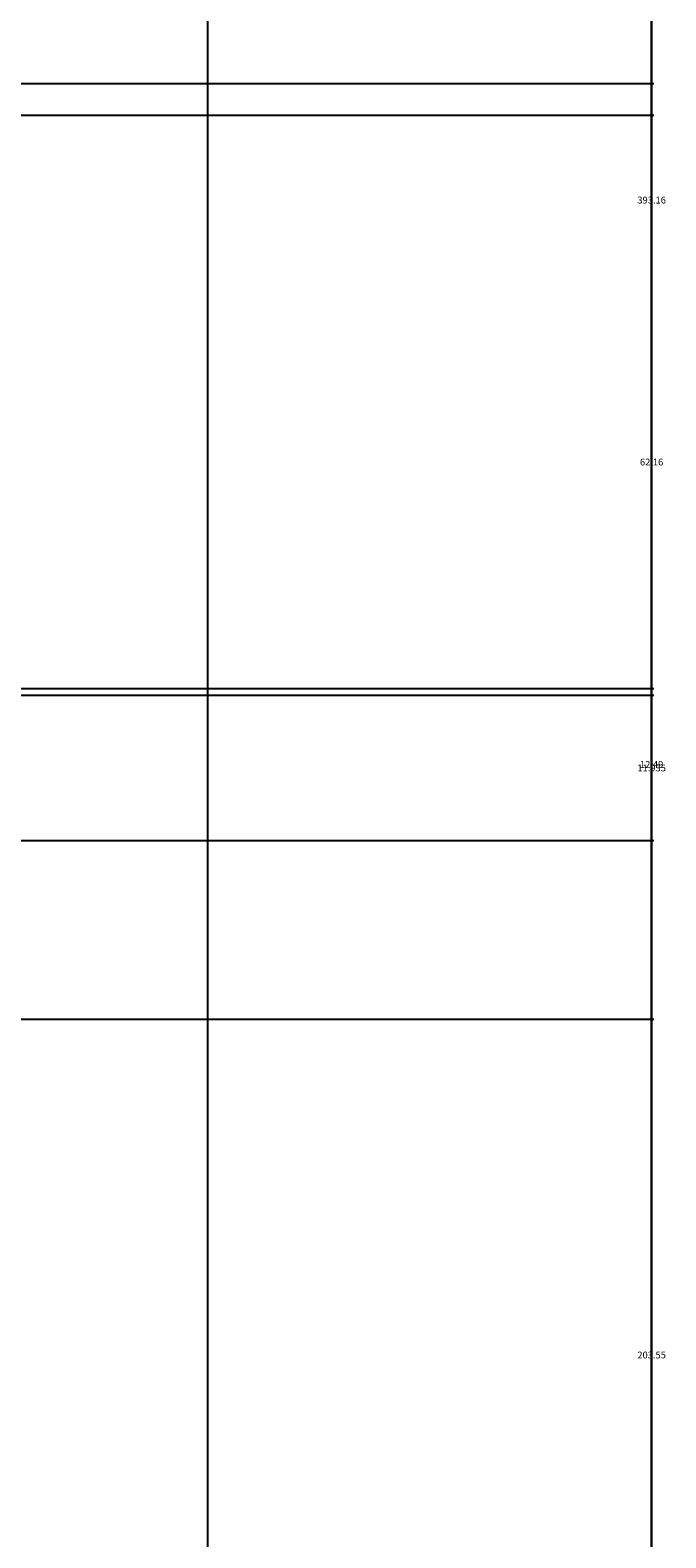
# Model space of a CAD drawing. Units: inches. Extents: x -26 to 776, y -22 to 650.
# Tile 55 of 62: x 724 to 776, y 102 to 226. Entities that reach past the tile are written whole.
import ezdxf

# ---------------------------------------------------------------- set-up
doc = ezdxf.new("R2010")
doc.units = ezdxf.units.IN
doc.header["$MEASUREMENT"] = 0
doc.layers.add('A-ANNO-DIMS', color=2, linetype='Continuous', lineweight=18)
doc.styles.get("Standard").update_dxf_attribs({"font": 'arial.ttf'})
doc.dimstyles.get("Standard").update_dxf_attribs({"dimtxt": 0.5625, "dimasz": 0.18, "dimexe": 0.18, "dimexo": 0.0625, "dimgap": 0.09, "dimtad": 0, "dimtih": 1, "dimtoh": 1, "dimdec": 4, "dimzin": 0, "dimdsep": 46, "dimlunit": 4, "dimtxsty": 'Standard', "dimcen": 0.09, "dimadec": 0, "dimazin": 0, "dimtfac": 1, "dimtdec": 4, "dimtofl": 0, "dimtmove": 0, "dimatfit": 3, "dimfxl": 1, "dimtolj": 1, "dimtzin": 0, "dimarcsym": 0})

# ---------------------------------------------------------------- blocks, each defined once
blk = doc.blocks.new('*D20')
at = {"layer": 'A-ANNO-DIMS', "color": 0, "lineweight": -2, "transparency": 16777216}
for p, q in [((425.81, 455.47), (775.34, 455.47)), ((775.16, 455.29), (775.16, 235.85)), ((775.16, 15.66), (775.16, 235.1)), ((425.81, 15.48), (775.34, 15.48))]:
    blk.add_line(p, q, dxfattribs=at)
at = {"layer": 'A-ANNO-DIMS', "color": 0, "transparency": 16777216}
for points in [[(775.13, 455.29), (775.19, 455.29), (775.16, 455.47)], [(775.13, 15.66), (775.19, 15.66), (775.16, 15.48)]]:
    blk.add_solid(points, dxfattribs=at)
at = {"layer": 'Defpoints', "color": 0, "transparency": 16777216}
for p in [(425.74, 455.47), (775.16, 455.47), (425.74, 15.48)]:
    blk.add_point(p, dxfattribs=at)
at = {"layer": 'A-ANNO-DIMS', "color": 0, "transparency": 16777216, "insert": (775.16, 235.48), "char_height": 0.562, "attachment_point": 5}
blk.add_mtext('\\A1;440', dxfattribs=at)
blk = doc.blocks.new('*D26')
at = {"layer": 'A-ANNO-DIMS', "color": 0, "lineweight": -2, "transparency": 16777216}
for p, q in [((91.71, 171.97), (775.34, 171.97)), ((775.16, 171.79), (775.16, 166.11)), ((775.16, 159.66), (775.16, 165.35)), ((82.2, 159.48), (775.34, 159.48))]:
    blk.add_line(p, q, dxfattribs=at)
at = {"layer": 'A-ANNO-DIMS', "color": 0, "transparency": 16777216}
for points in [[(775.13, 171.79), (775.19, 171.79), (775.16, 171.97)], [(775.13, 159.66), (775.19, 159.66), (775.16, 159.48)]]:
    blk.add_solid(points, dxfattribs=at)
at = {"layer": 'Defpoints', "color": 0, "transparency": 16777216}
for p in [(91.64, 171.97), (775.16, 171.97), (82.13, 159.48)]:
    blk.add_point(p, dxfattribs=at)
at = {"layer": 'A-ANNO-DIMS', "color": 0, "transparency": 16777216, "insert": (775.16, 165.73), "char_height": 0.562, "attachment_point": 5}
blk.add_mtext('\\A1;12.49', dxfattribs=at)
blk = doc.blocks.new('*D28')
at = {"layer": 'A-ANNO-DIMS', "color": 0, "lineweight": -2, "transparency": 16777216}
for p, q in [((285.08, 314.12), (775.34, 314.12)), ((775.16, 313.94), (775.16, 243.14)), ((775.16, 171.6), (775.16, 242.4)), ((285.08, 171.42), (775.34, 171.42))]:
    blk.add_line(p, q, dxfattribs=at)
at = {"layer": 'A-ANNO-DIMS', "color": 0, "transparency": 16777216}
for points in [[(775.13, 313.94), (775.19, 313.94), (775.16, 314.12)], [(775.13, 171.6), (775.19, 171.6), (775.16, 171.42)]]:
    blk.add_solid(points, dxfattribs=at)
at = {"layer": 'Defpoints', "color": 0, "transparency": 16777216}
for p in [(285.02, 314.12), (775.16, 314.12), (285.02, 171.42)]:
    blk.add_point(p, dxfattribs=at)
at = {"layer": 'A-ANNO-DIMS', "color": 0, "transparency": 16777216, "insert": (775.16, 242.77), "char_height": 0.562, "attachment_point": 5}
blk.add_mtext('\\A1;142.7', dxfattribs=at)
blk = doc.blocks.new('*D30')
at = {"layer": 'A-ANNO-DIMS', "color": 0, "lineweight": -2, "transparency": 16777216}
for p, q in [((280.68, 144.84), (775.34, 144.84)), ((775.16, 144.66), (775.16, 86.01)), ((775.16, 26.6), (775.16, 85.25)), ((280.68, 26.42), (775.34, 26.42))]:
    blk.add_line(p, q, dxfattribs=at)
at = {"layer": 'A-ANNO-DIMS', "color": 0, "transparency": 16777216}
for points in [[(775.13, 144.66), (775.19, 144.66), (775.16, 144.84)], [(775.13, 26.6), (775.19, 26.6), (775.16, 26.42)]]:
    blk.add_solid(points, dxfattribs=at)
at = {"layer": 'Defpoints', "color": 0, "transparency": 16777216}
for p in [(280.62, 144.84), (775.16, 144.84), (280.62, 26.42)]:
    blk.add_point(p, dxfattribs=at)
at = {"layer": 'A-ANNO-DIMS', "color": 0, "transparency": 16777216, "insert": (775.16, 85.63), "char_height": 0.562, "attachment_point": 5}
blk.add_mtext('\\A1;118.41', dxfattribs=at)
blk = doc.blocks.new('*D41')
at = {"layer": 'A-ANNO-DIMS', "color": 0, "lineweight": -2, "transparency": 16777216}
for p, q in [((11.17, 221.64), (775.34, 221.64)), ((775.16, 221.46), (775.16, 190.94)), ((775.16, 159.66), (775.16, 190.18)), ((11.17, 159.48), (775.34, 159.48))]:
    blk.add_line(p, q, dxfattribs=at)
at = {"layer": 'A-ANNO-DIMS', "color": 0, "transparency": 16777216}
for points in [[(775.13, 221.46), (775.19, 221.46), (775.16, 221.64)], [(775.13, 159.66), (775.19, 159.66), (775.16, 159.48)]]:
    blk.add_solid(points, dxfattribs=at)
at = {"layer": 'Defpoints', "color": 0, "transparency": 16777216}
for p in [(11.11, 221.64), (775.16, 221.64), (11.11, 159.48)]:
    blk.add_point(p, dxfattribs=at)
at = {"layer": 'A-ANNO-DIMS', "color": 0, "transparency": 16777216, "insert": (775.16, 190.56), "char_height": 0.562, "attachment_point": 5}
blk.add_mtext('\\A1;62.16', dxfattribs=at)
blk = doc.blocks.new('*D42')
at = {"layer": 'A-ANNO-DIMS', "color": 0, "lineweight": -2, "transparency": 16777216}
for p, q in [((285.08, 171.42), (775.34, 171.42)), ((775.16, 171.24), (775.16, 165.83)), ((775.16, 159.66), (775.16, 165.07)), ((289.3, 159.48), (775.34, 159.48))]:
    blk.add_line(p, q, dxfattribs=at)
at = {"layer": 'A-ANNO-DIMS', "color": 0, "transparency": 16777216}
for points in [[(775.13, 171.24), (775.19, 171.24), (775.16, 171.42)], [(775.13, 159.66), (775.19, 159.66), (775.16, 159.48)]]:
    blk.add_solid(points, dxfattribs=at)
at = {"layer": 'Defpoints', "color": 0, "transparency": 16777216}
for p in [(285.02, 171.42), (775.16, 171.42), (289.24, 159.48)]:
    blk.add_point(p, dxfattribs=at)
at = {"layer": 'A-ANNO-DIMS', "color": 0, "transparency": 16777216, "insert": (775.16, 165.45), "char_height": 0.562, "attachment_point": 5}
blk.add_mtext('\\A1;11.935', dxfattribs=at)
blk = doc.blocks.new('*D45')
at = {"layer": 'A-ANNO-DIMS', "color": 0, "lineweight": -2, "transparency": 16777216}
for p, q in [((507.74, 408.64), (775.34, 408.64)), ((775.16, 408.46), (775.16, 212.44)), ((775.16, 15.66), (775.16, 211.68)), ((586, 15.48), (775.34, 15.48))]:
    blk.add_line(p, q, dxfattribs=at)
at = {"layer": 'A-ANNO-DIMS', "color": 0, "transparency": 16777216}
for points in [[(775.13, 408.46), (775.19, 408.46), (775.16, 408.64)], [(775.13, 15.66), (775.19, 15.66), (775.16, 15.48)]]:
    blk.add_solid(points, dxfattribs=at)
at = {"layer": 'Defpoints', "color": 0, "transparency": 16777216}
for p in [(507.68, 408.64), (775.16, 408.64), (585.94, 15.48)]:
    blk.add_point(p, dxfattribs=at)
at = {"layer": 'A-ANNO-DIMS', "color": 0, "transparency": 16777216, "insert": (775.16, 212.06), "char_height": 0.562, "attachment_point": 5}
blk.add_mtext('\\A1;393.16', dxfattribs=at)
blk = doc.blocks.new('*D46')
at = {"layer": 'A-ANNO-DIMS', "color": 0, "lineweight": -2, "transparency": 16777216}
for p, q in [((658.51, 219.03), (775.34, 219.03)), ((775.16, 218.85), (775.16, 117.63)), ((775.16, 15.66), (775.16, 116.88)), ((677.97, 15.48), (775.34, 15.48))]:
    blk.add_line(p, q, dxfattribs=at)
at = {"layer": 'A-ANNO-DIMS', "color": 0, "transparency": 16777216}
for points in [[(775.13, 218.85), (775.19, 218.85), (775.16, 219.03)], [(775.13, 15.66), (775.19, 15.66), (775.16, 15.48)]]:
    blk.add_solid(points, dxfattribs=at)
at = {"layer": 'Defpoints', "color": 0, "transparency": 16777216}
for p in [(658.44, 219.03), (775.16, 219.03), (677.9, 15.48)]:
    blk.add_point(p, dxfattribs=at)
at = {"layer": 'A-ANNO-DIMS', "color": 0, "transparency": 16777216, "insert": (775.16, 117.26), "char_height": 0.562, "attachment_point": 5}
blk.add_mtext('\\A1;203.55', dxfattribs=at)
blk = doc.blocks.new('*D48')
at = {"layer": 'A-ANNO-DIMS', "color": 0, "lineweight": -2, "transparency": 16777216}
for p, q in [((545.03, 67.41), (545.03, 649.86)), ((738.75, 50.91), (738.75, 649.86)), ((545.21, 649.68), (640.88, 649.68)), ((738.57, 649.68), (642.9, 649.68))]:
    blk.add_line(p, q, dxfattribs=at)
at = {"layer": 'A-ANNO-DIMS', "color": 0, "transparency": 16777216}
for points in [[(545.21, 649.71), (545.21, 649.65), (545.03, 649.68)], [(738.57, 649.71), (738.57, 649.65), (738.75, 649.68)]]:
    blk.add_solid(points, dxfattribs=at)
at = {"layer": 'Defpoints', "color": 0, "transparency": 16777216}
for p in [(738.75, 649.68), (545.03, 67.35), (738.75, 50.85)]:
    blk.add_point(p, dxfattribs=at)
at = {"layer": 'A-ANNO-DIMS', "color": 0, "transparency": 16777216, "insert": (641.89, 649.68), "char_height": 0.562, "attachment_point": 5}
blk.add_mtext('\\A1;193.7', dxfattribs=at)

msp = doc.modelspace()

# ---------------------------------------------------------------- dimensions: what is measured, and where the dimension line sits
at = {"layer": 'A-ANNO-DIMS'}
dim = msp.add_linear_dim(base=(738.7503, 649.6763), p1=(545.0331, 67.3523), p2=(738.7503, 50.8482), dimstyle='Standard', override={"dimdec": 1, "dimlfac": 1, "dimrnd": 0, "dimzin": 0, "dimdsep": 46, "dimlunit": 2}, dxfattribs=at)
dim.commit()
dim.dimension.update_dxf_attribs({"geometry": '*D48', "text_midpoint": (641.8917, 649.6763)})
for base, p1, p2, override, picture, middle in [((775.1553, 455.4717), (425.7434, 15.4824), (425.7434, 455.4717), {"dimdec": 0, "dimlfac": 1, "dimrnd": 0, "dimzin": 0, "dimdsep": 46, "dimlunit": 2}, '*D20', (775.1553, 235.477)), ((775.1553, 408.6389), (585.9354, 15.4824), (507.6759, 408.6389), {"dimdec": 2, "dimlfac": 1, "dimrnd": 0, "dimzin": 0, "dimdsep": 46, "dimlunit": 2}, '*D45', (775.1553, 212.0606)), ((775.1553, 314.119), (285.0179, 171.4173), (285.0179, 314.119), {"dimdec": 1, "dimlfac": 1, "dimrnd": 0, "dimzin": 0, "dimdsep": 46, "dimlunit": 2}, '*D28', (775.1553, 242.7682)), ((775.1553, 221.6413), (11.1074, 159.4824), (11.1074, 221.6413), {"dimdec": 2, "dimlfac": 1, "dimrnd": 0, "dimzin": 0, "dimdsep": 46, "dimlunit": 2}, '*D41', (775.1553, 190.5618)), ((775.1553, 219.0324), (677.9037, 15.4824), (658.4435, 219.0324), {"dimdec": 2, "dimlfac": 1, "dimrnd": 0, "dimzin": 0, "dimdsep": 46, "dimlunit": 2}, '*D46', (775.1553, 117.2574)), ((775.1553, 171.9734), (82.134, 159.4824), (91.6448, 171.9734), {"dimdec": 2, "dimlfac": 1, "dimrnd": 0, "dimzin": 0, "dimdsep": 46, "dimlunit": 2}, '*D26', (775.1553, 165.7279)), ((775.1553, 171.4173), (289.2424, 159.4824), (285.0179, 171.4173), {"dimdec": 3, "dimlfac": 1, "dimrnd": 0, "dimzin": 0, "dimdsep": 46, "dimlunit": 2}, '*D42', (775.1553, 165.4498)), ((775.1553, 144.8359), (280.6173, 26.4239), (280.6173, 144.8359), {"dimdec": 2, "dimlfac": 1, "dimrnd": 0, "dimzin": 0, "dimdsep": 46, "dimlunit": 2}, '*D30', (775.1553, 85.6299))]:
    dim = msp.add_linear_dim(base=base, p1=p1, p2=p2, angle=90, dimstyle='Standard', override=override, dxfattribs=at)
    dim.commit()
    dim.dimension.update_dxf_attribs({"geometry": picture, "text_midpoint": middle})

doc.saveas('drawing.dxf')
